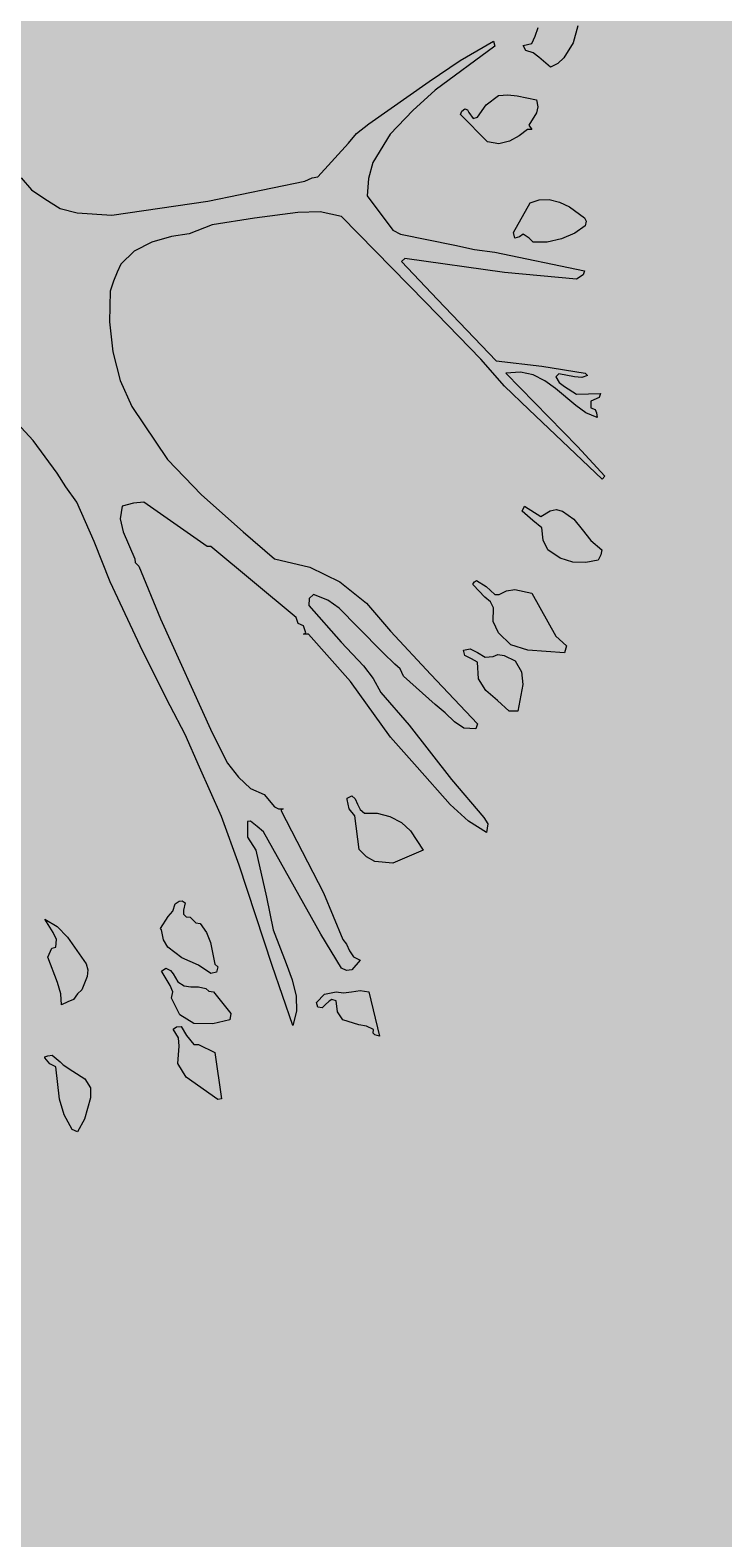
# Model space of a CAD drawing. Units: inches. Extents: x 84 to 1044, y -280 to 906.
# Tile 58 of 105: x 401.24 to 411.62, y 738.5 to 761.07. Entities that reach past the tile are written whole.
import ezdxf

# ---------------------------------------------------------------- set-up
doc = ezdxf.new("R2010")
doc.units = ezdxf.units.IN
doc.layers.add('A-ANNO-DIMS', color=2, linetype='Continuous', lineweight=18)
doc.layers.add('L-PLNT', color=114, linetype='Continuous', lineweight=15)
doc.layers.add('L-PLNT-PATT', color=9, linetype='Continuous', lineweight=9, true_color=0xafd9aa)
doc.styles.get("Standard").update_dxf_attribs({"font": 'arial.ttf'})
doc.dimstyles.get("Standard").update_dxf_attribs({"dimtxt": 0.18, "dimasz": 0.18, "dimexe": 0.18, "dimexo": 0.0625, "dimgap": 0.09, "dimtad": 0, "dimtih": 1, "dimtoh": 1, "dimdec": 4, "dimzin": 0, "dimdsep": 46, "dimtxsty": 'Standard', "dimcen": 0.09, "dimadec": 0, "dimazin": 0, "dimtfac": 1, "dimtdec": 4, "dimtofl": 0, "dimtmove": 0, "dimatfit": 3, "dimfxl": 1, "dimtolj": 1, "dimtzin": 0, "dimarcsym": 0})

# ---------------------------------------------------------------- blocks, each defined once
blk = doc.blocks.new('A$C37E508DF')
for p, q in [((1.3455, 1.0934), (1.3485, 1.102)), ((1.3875, 1.1037), (1.3828, 1.087)), ((1.2713, 1.0694), (1.3044, 1.0887)), ((1.3044, 1.0887), (1.3057, 1.0835)), ((1.3335, 1.0844), (1.3421, 1.0861)), ((1.3421, 1.0861), (1.3455, 1.0934)), ((1.3828, 1.087), (1.3738, 1.072)), ((1.3057, 1.0835), (1.2469, 1.0402)), ((1.3361, 1.0793), (1.3335, 1.0844)), ((1.3434, 1.0771), (1.3361, 1.0793)), ((1.349, 1.0728), (1.3434, 1.0771)), ((1.3605, 1.063), (1.349, 1.0728)), ((1.3738, 1.072), (1.3678, 1.0664)), ((1.2409, 1.0488), (1.2713, 1.0694)), ((1.3678, 1.0664), (1.3605, 1.063)), ((1.1813, 1.0072), (1.2409, 1.0488)), ((1.2469, 1.0402), (1.2246, 1.0201)), ((1.2885, 1.0136), (1.2971, 1.0257)), ((1.2971, 1.0257), (1.3091, 1.0351)), ((1.3091, 1.0351), (1.3185, 1.0355)), ((1.3185, 1.0355), (1.3275, 1.0347)), ((1.3275, 1.0347), (1.3468, 1.0308)), ((1.3468, 1.0308), (1.3481, 1.0239)), ((1.2246, 1.0201), (1.2023, 0.9969)), ((1.2718, 1.0162), (1.2731, 1.0197)), ((1.2984, 0.9892), (1.2718, 1.0162)), ((1.2731, 1.0197), (1.2761, 1.0218)), ((1.2761, 1.0218), (1.2786, 1.0209)), ((1.2786, 1.0209), (1.2799, 1.0184)), ((1.2799, 1.0184), (1.2842, 1.0124)), ((1.2842, 1.0124), (1.2885, 1.0136)), ((1.3468, 1.018), (1.3391, 1.0059)), ((1.3481, 1.0239), (1.3468, 1.018)), ((1.1612, 0.9879), (1.1693, 0.9974)), ((1.1693, 0.9974), (1.1813, 1.0072)), ((1.2023, 0.9969), (1.1852, 0.9691)), ((1.3378, 1.0016), (1.3297, 0.9952)), ((1.3421, 1.0016), (1.3378, 1.0016)), ((1.3391, 1.0059), (1.3421, 1.0016)), ((1.1311, 0.9549), (1.1612, 0.9879)), ((1.3095, 0.9875), (1.2984, 0.9892)), ((1.3202, 0.9901), (1.3095, 0.9875)), ((1.3297, 0.9952), (1.3202, 0.9901)), ((1.1852, 0.9691), (1.1809, 0.9532)), ((0.8383, 0.954), (0.8486, 0.942)), ((1.1183, 0.9506), (1.1256, 0.954)), ((1.1256, 0.954), (1.1311, 0.9549)), ((1.1809, 0.9532), (1.1796, 0.936)), ((0.8486, 0.942), (0.8619, 0.933)), ((1.0227, 0.9309), (1.1183, 0.9506)), ((0.8619, 0.933), (0.8769, 0.9236)), ((0.8769, 0.9236), (0.8936, 0.9193)), ((0.9279, 0.9172), (1.0227, 0.9309)), ((1.1796, 0.936), (1.2049, 0.9022)), ((1.3241, 0.9), (1.3404, 0.9292)), ((1.3404, 0.9292), (1.3494, 0.9322)), ((1.3494, 0.9322), (1.3592, 0.9326)), ((1.3592, 0.9326), (1.3695, 0.93)), ((1.3695, 0.93), (1.3794, 0.9253)), ((1.3794, 0.9253), (1.394, 0.9146)), ((0.8936, 0.9193), (0.9279, 0.9172)), ((1.0269, 0.9077), (1.0042, 0.8987)), ((1.0685, 0.9142), (1.0269, 0.9077)), ((1.1114, 0.9198), (1.0685, 0.9142)), ((1.1333, 0.9202), (1.1114, 0.9198)), ((1.1543, 0.9159), (1.1333, 0.9202)), ((1.2371, 0.8314), (1.1543, 0.9159)), ((1.3948, 0.9065), (1.3846, 0.8992)), ((1.394, 0.9146), (1.3957, 0.9112)), ((1.3957, 0.9112), (1.3948, 0.9065)), ((0.9866, 0.8962), (0.9673, 0.8906)), ((1.0042, 0.8987), (0.9866, 0.8962)), ((1.2049, 0.9022), (1.2126, 0.8983)), ((1.2126, 0.8983), (1.2662, 0.8876)), ((1.3254, 0.8944), (1.3241, 0.9)), ((1.3301, 0.8957), (1.3254, 0.8944)), ((1.3335, 0.8983), (1.3301, 0.8957)), ((1.3395, 0.8944), (1.3335, 0.8983)), ((1.3434, 0.8906), (1.3395, 0.8944)), ((1.3713, 0.8936), (1.3571, 0.8906)), ((1.3846, 0.8992), (1.3713, 0.8936)), ((0.9498, 0.8816), (0.9369, 0.8687)), ((0.9673, 0.8906), (0.9498, 0.8816)), ((1.2662, 0.8876), (1.2855, 0.8833)), ((1.2855, 0.8833), (1.3057, 0.8807)), ((1.3057, 0.8807), (1.394, 0.8623)), ((1.3571, 0.8906), (1.3434, 0.8906)), ((0.9369, 0.8687), (0.933, 0.861)), ((1.2169, 0.8743), (1.2135, 0.8713)), ((1.2135, 0.8713), (1.2491, 0.834)), ((1.3151, 0.8606), (1.2169, 0.8743)), ((1.394, 0.8623), (1.3927, 0.8584)), ((0.9296, 0.852), (0.9262, 0.8421)), ((0.933, 0.861), (0.9296, 0.852)), ((1.3863, 0.8541), (1.3151, 0.8606)), ((1.3927, 0.8584), (1.3863, 0.8541)), ((0.9262, 0.8421), (0.9257, 0.8121)), ((1.2491, 0.834), (1.3069, 0.7735)), ((1.2919, 0.7752), (1.2371, 0.8314)), ((0.9257, 0.8121), (0.9287, 0.7825)), ((0.9287, 0.7825), (0.936, 0.7542)), ((1.3151, 0.7487), (1.2919, 0.7752)), ((1.3069, 0.7735), (1.352, 0.7684)), ((1.3309, 0.7624), (1.3164, 0.7615)), ((1.3164, 0.7615), (1.3871, 0.6891)), ((1.3434, 0.7598), (1.3309, 0.7624)), ((1.355, 0.7538), (1.3434, 0.7598)), ((1.352, 0.7684), (1.3948, 0.7615)), ((1.3687, 0.7607), (1.3657, 0.7577)), ((1.3841, 0.7577), (1.3687, 0.7607)), ((1.397, 0.759), (1.3914, 0.7572)), ((1.3948, 0.7615), (1.397, 0.759)), ((0.936, 0.7542), (0.9476, 0.7285)), ((1.3391, 0.7255), (1.3151, 0.7487)), ((1.3653, 0.7461), (1.355, 0.7538)), ((1.3854, 0.7294), (1.3653, 0.7461)), ((1.3657, 0.7577), (1.3691, 0.7521)), ((1.3691, 0.7521), (1.3743, 0.7482)), ((1.3743, 0.7482), (1.3863, 0.7405)), ((1.3914, 0.7572), (1.3841, 0.7577)), ((0.9476, 0.7285), (0.9828, 0.6762)), ((1.3953, 0.7221), (1.3854, 0.7294)), ((1.3863, 0.7405), (1.4099, 0.7414)), ((1.4086, 0.7375), (1.4004, 0.7337)), ((1.4004, 0.7337), (1.4004, 0.7272)), ((1.4099, 0.7414), (1.4086, 0.7375)), ((1.4116, 0.6569), (1.3391, 0.7255)), ((1.4064, 0.7178), (1.3953, 0.7221)), ((1.4004, 0.7272), (1.4047, 0.7255)), ((1.4047, 0.7255), (1.406, 0.7221)), ((1.406, 0.7221), (1.4064, 0.7178)), ((0.8503, 0.6951), (0.8344, 0.7122)), ((0.8739, 0.6629), (0.8503, 0.6951)), ((1.3871, 0.6891), (1.4141, 0.6599)), ((0.9828, 0.6762), (1.0162, 0.6415)), ((0.8824, 0.6492), (0.8739, 0.6629)), ((1.4141, 0.6599), (1.4116, 0.6569)), ((0.8932, 0.6342), (0.8824, 0.6492)), ((1.0162, 0.6415), (1.0574, 0.605)), ((0.9103, 0.5956), (0.8932, 0.6342)), ((0.9382, 0.6303), (0.936, 0.6179)), ((0.9493, 0.6333), (0.9382, 0.6303)), ((0.9596, 0.6342), (0.9493, 0.6333)), ((1.0218, 0.5904), (0.9596, 0.6342)), ((1.3327, 0.6252), (1.3348, 0.6303)), ((1.343, 0.6162), (1.3327, 0.6252)), ((1.3348, 0.6303), (1.3511, 0.62)), ((1.3511, 0.62), (1.3601, 0.6256)), ((1.3601, 0.6256), (1.3661, 0.6269)), ((1.3661, 0.6269), (1.3725, 0.6252)), ((1.3725, 0.6252), (1.3837, 0.6175)), ((0.936, 0.6179), (0.939, 0.605)), ((1.352, 0.6089), (1.343, 0.6162)), ((1.3837, 0.6175), (1.3918, 0.6072)), ((0.9262, 0.5557), (0.9103, 0.5956)), ((0.939, 0.605), (0.9506, 0.5784)), ((1.0574, 0.605), (1.0883, 0.5784)), ((1.3533, 0.5969), (1.352, 0.6089)), ((1.358, 0.5874), (1.3533, 0.5969)), ((1.3918, 0.6072), (1.4004, 0.5964)), ((1.4004, 0.5964), (1.4111, 0.5874)), ((1.0256, 0.5904), (1.0218, 0.5904)), ((1.1097, 0.5205), (1.0256, 0.5904)), ((1.37, 0.5789), (1.358, 0.5874)), ((1.4103, 0.5823), (1.4077, 0.5771)), ((1.4111, 0.5874), (1.4103, 0.5823)), ((0.9506, 0.5784), (0.951, 0.5746)), ((0.951, 0.5746), (0.9545, 0.5711)), ((0.9545, 0.5711), (0.9759, 0.5193)), ((1.0883, 0.5784), (1.123, 0.5703)), ((1.123, 0.5703), (1.1526, 0.5557)), ((1.3824, 0.575), (1.37, 0.5789)), ((1.3953, 0.5746), (1.3824, 0.575)), ((1.4077, 0.5771), (1.3953, 0.5746)), ((0.9583, 0.4871), (0.9262, 0.5557)), ((1.1526, 0.5557), (1.1792, 0.5347)), ((1.2842, 0.554), (1.2855, 0.5557)), ((1.2842, 0.5527), (1.2842, 0.554)), ((1.2958, 0.5407), (1.2842, 0.5527)), ((1.2855, 0.5557), (1.2876, 0.557)), ((1.2876, 0.557), (1.2971, 0.551)), ((1.2971, 0.551), (1.3057, 0.5433)), ((1.1226, 0.5394), (1.1221, 0.5325)), ((1.1268, 0.5433), (1.1226, 0.5394)), ((1.141, 0.5377), (1.1268, 0.5433)), ((1.1521, 0.5296), (1.141, 0.5377)), ((1.3014, 0.536), (1.2958, 0.5407)), ((1.3044, 0.53), (1.3014, 0.536)), ((1.3057, 0.5433), (1.3099, 0.5433)), ((1.3099, 0.5433), (1.3172, 0.5467)), ((1.3172, 0.5467), (1.3254, 0.548)), ((1.3254, 0.548), (1.3421, 0.5446)), ((1.3421, 0.5446), (1.3657, 0.5021)), ((1.1118, 0.5145), (1.1097, 0.5205)), ((1.1221, 0.5325), (1.1539, 0.4961)), ((1.1706, 0.5111), (1.1521, 0.5296)), ((1.1792, 0.5347), (1.2027, 0.5072)), ((1.3039, 0.5167), (1.3044, 0.53)), ((0.9759, 0.5193), (1.0269, 0.4069)), ((1.117, 0.5124), (1.1118, 0.5145)), ((1.1191, 0.5055), (1.117, 0.5124)), ((1.117, 0.5042), (1.1191, 0.5055)), ((1.1955, 0.4858), (1.1706, 0.5111)), ((1.2027, 0.5072), (1.2426, 0.4644)), ((1.3091, 0.5055), (1.3039, 0.5167)), ((1.3215, 0.4935), (1.3091, 0.5055)), ((1.1217, 0.5042), (1.117, 0.5042)), ((1.1633, 0.4575), (1.1217, 0.5042)), ((1.1539, 0.4961), (1.1762, 0.4729)), ((1.3382, 0.4884), (1.3215, 0.4935)), ((1.3657, 0.5021), (1.3764, 0.4927)), ((1.3764, 0.4927), (1.3743, 0.4858)), ((0.9853, 0.4335), (0.9583, 0.4871)), ((1.207, 0.4747), (1.1955, 0.4858)), ((1.2748, 0.4884), (1.2812, 0.4897)), ((1.2761, 0.4832), (1.2748, 0.4884)), ((1.2825, 0.4798), (1.2761, 0.4832)), ((1.2812, 0.4897), (1.2885, 0.4862)), ((1.2885, 0.4764), (1.2825, 0.4798)), ((1.2885, 0.4862), (1.2962, 0.4815)), ((1.2894, 0.4601), (1.2885, 0.4764)), ((1.2962, 0.4815), (1.3039, 0.482)), ((1.3039, 0.482), (1.3087, 0.4841)), ((1.3087, 0.4841), (1.3147, 0.4832)), ((1.3147, 0.4832), (1.3258, 0.4777)), ((1.3258, 0.4777), (1.3318, 0.4669)), ((1.3743, 0.4858), (1.3382, 0.4884)), ((1.1762, 0.4729), (1.1856, 0.4605)), ((1.2122, 0.47), (1.207, 0.4747)), ((1.2156, 0.4627), (1.2122, 0.47)), ((1.2469, 0.4348), (1.2156, 0.4627)), ((1.2426, 0.4644), (1.2885, 0.4159)), ((1.3318, 0.4669), (1.3331, 0.4545)), ((1.2027, 0.4026), (1.1633, 0.4575)), ((1.1856, 0.4605), (1.1933, 0.4468)), ((1.1933, 0.4468), (1.2212, 0.4146)), ((1.2967, 0.4485), (1.2894, 0.4601)), ((1.3082, 0.4386), (1.2967, 0.4485)), ((1.3331, 0.4545), (1.3284, 0.4284)), ((1.0003, 0.4052), (0.9853, 0.4335)), ((1.2568, 0.4266), (1.2469, 0.4348)), ((1.3198, 0.4284), (1.3082, 0.4386)), ((1.2658, 0.4176), (1.2568, 0.4266)), ((1.2752, 0.4116), (1.2658, 0.4176)), ((1.3284, 0.4284), (1.3198, 0.4284)), ((1.0145, 0.373), (1.0003, 0.4052)), ((1.0269, 0.4069), (1.0419, 0.3769)), ((1.2289, 0.373), (1.2027, 0.4026)), ((1.2212, 0.4146), (1.2628, 0.361)), ((1.2868, 0.4108), (1.2752, 0.4116)), ((1.2885, 0.4159), (1.2868, 0.4108)), ((1.0359, 0.3246), (1.0145, 0.373)), ((1.0419, 0.3769), (1.0527, 0.3632)), ((1.2615, 0.3362), (1.2289, 0.373)), ((1.0527, 0.3632), (1.0647, 0.352)), ((1.2628, 0.361), (1.2949, 0.3233)), ((1.0647, 0.352), (1.078, 0.346)), ((1.078, 0.346), (1.0883, 0.334)), ((1.1599, 0.3426), (1.1646, 0.3447)), ((1.1599, 0.3413), (1.1599, 0.3426)), ((1.1646, 0.3447), (1.168, 0.3417)), ((1.0883, 0.334), (1.0921, 0.3319)), ((1.0921, 0.3319), (1.0968, 0.3319)), ((1.0968, 0.3319), (1.0947, 0.3306)), ((1.0947, 0.3306), (1.1367, 0.2491)), ((1.162, 0.3319), (1.1599, 0.3413)), ((1.1676, 0.325), (1.162, 0.3319)), ((1.168, 0.3417), (1.1702, 0.3366)), ((1.1702, 0.3366), (1.1727, 0.3314)), ((1.1727, 0.3314), (1.177, 0.3276)), ((1.177, 0.3276), (1.1895, 0.3276)), ((1.1895, 0.3276), (1.2019, 0.3246)), ((1.2795, 0.3199), (1.2615, 0.3362)), ((1.0535, 0.2766), (1.0359, 0.3246)), ((1.0647, 0.3199), (1.0617, 0.3194)), ((1.0617, 0.3194), (1.0617, 0.304)), ((1.0711, 0.3147), (1.0647, 0.3199)), ((1.0775, 0.3092), (1.0711, 0.3147)), ((1.1719, 0.292), (1.1676, 0.325)), ((1.2019, 0.3246), (1.2135, 0.3186)), ((1.2135, 0.3186), (1.2225, 0.3104)), ((1.2975, 0.3087), (1.2795, 0.3199)), ((1.2949, 0.3233), (1.2988, 0.3173)), ((1.2988, 0.3173), (1.2975, 0.3087)), ((1.0617, 0.304), (1.0698, 0.2911)), ((1.1341, 0.2084), (1.0775, 0.3092)), ((1.2225, 0.3104), (1.2349, 0.2911)), ((1.0698, 0.2911), (1.0805, 0.2448)), ((1.1792, 0.2847), (1.1719, 0.292)), ((1.1873, 0.28), (1.1792, 0.2847)), ((1.2349, 0.2911), (1.2049, 0.2783)), ((1.0861, 0.1775), (1.0535, 0.2766)), ((1.2049, 0.2783), (1.1873, 0.28)), ((0.9879, 0.2311), (0.9905, 0.2384)), ((0.9905, 0.2384), (0.9943, 0.241)), ((0.9943, 0.241), (0.9973, 0.2414)), ((0.9973, 0.2414), (1.0003, 0.2393)), ((1.0003, 0.2393), (0.9986, 0.232)), ((1.0805, 0.2448), (1.087, 0.2127)), ((1.1367, 0.2491), (1.1556, 0.2032)), ((0.8619, 0.2234), (0.8739, 0.2161)), ((0.87, 0.2101), (0.8619, 0.2234)), ((0.9759, 0.214), (0.9836, 0.226)), ((0.9836, 0.226), (0.9879, 0.2311)), ((0.9986, 0.232), (0.9986, 0.2281)), ((0.9986, 0.2281), (1.0012, 0.2255)), ((1.0012, 0.2255), (1.0051, 0.2251)), ((1.0051, 0.2251), (1.0076, 0.2225)), ((0.8734, 0.2032), (0.87, 0.2101)), ((0.8739, 0.2161), (0.8841, 0.2054)), ((0.9768, 0.2127), (0.9759, 0.214)), ((0.9789, 0.2028), (0.9768, 0.2127)), ((1.0076, 0.2225), (1.0106, 0.2195)), ((1.0106, 0.2195), (1.0149, 0.2191)), ((1.0149, 0.2191), (1.0214, 0.2101)), ((1.0214, 0.2101), (1.0252, 0.2002)), ((1.087, 0.2127), (1.0998, 0.1797)), ((1.1543, 0.1749), (1.1341, 0.2084)), ((0.8649, 0.1857), (0.8687, 0.1947)), ((0.8687, 0.1947), (0.8726, 0.1955)), ((0.8726, 0.1955), (0.8734, 0.2032)), ((0.8841, 0.2054), (0.9026, 0.1792)), ((0.9832, 0.1955), (0.9789, 0.2028)), ((0.9969, 0.1852), (0.9832, 0.1955)), ((1.0252, 0.2002), (1.0295, 0.1788)), ((1.1556, 0.2032), (1.1594, 0.1985)), ((1.1594, 0.1985), (1.1624, 0.1921)), ((0.8743, 0.1608), (0.8649, 0.1857)), ((0.9026, 0.1792), (0.9043, 0.1732)), ((1.0132, 0.1779), (0.9969, 0.1852)), ((1.0295, 0.1788), (1.0325, 0.1762)), ((1.0998, 0.1797), (1.1058, 0.1634)), ((1.1624, 0.1921), (1.1663, 0.1861)), ((1.1727, 0.1827), (1.1646, 0.1732)), ((1.1663, 0.1861), (1.1727, 0.1827)), ((0.9035, 0.1668), (0.8983, 0.1535)), ((0.9043, 0.1732), (0.9035, 0.1668)), ((0.9768, 0.1719), (0.9811, 0.1749)), ((0.9776, 0.1711), (0.9768, 0.1719)), ((0.9853, 0.1578), (0.9776, 0.1711)), ((0.9811, 0.1749), (0.9858, 0.1728)), ((0.9858, 0.1728), (0.9884, 0.1694)), ((0.9884, 0.1694), (0.9931, 0.1616)), ((1.0256, 0.1698), (1.0132, 0.1779)), ((1.0312, 0.1711), (1.0256, 0.1698)), ((1.0325, 0.1762), (1.0312, 0.1711)), ((1.1063, 0.1183), (1.0861, 0.1775)), ((1.1594, 0.1728), (1.1543, 0.1749)), ((1.1646, 0.1732), (1.1594, 0.1728)), ((0.8777, 0.1496), (0.8743, 0.1608)), ((0.8781, 0.1389), (0.8777, 0.1496)), ((0.894, 0.1496), (0.8902, 0.1441)), ((0.8983, 0.1535), (0.894, 0.1496)), ((0.9879, 0.1518), (0.9853, 0.1578)), ((0.9866, 0.1453), (0.9879, 0.1518)), ((0.9931, 0.1616), (0.9991, 0.1574)), ((0.9991, 0.1574), (1.0059, 0.1565)), ((1.0059, 0.1565), (1.0132, 0.1565)), ((1.0132, 0.1565), (1.0205, 0.1548)), ((1.0205, 0.1548), (1.0235, 0.1522)), ((1.0235, 0.1522), (1.0282, 0.1518)), ((1.0282, 0.1518), (1.0454, 0.1303)), ((1.1058, 0.1634), (1.1097, 0.1475)), ((1.1298, 0.1411), (1.1376, 0.1492)), ((1.1376, 0.1492), (1.1491, 0.1518)), ((1.1491, 0.1518), (1.1564, 0.1505)), ((1.1564, 0.1505), (1.1642, 0.1518)), ((1.1642, 0.1518), (1.1727, 0.1531)), ((1.1727, 0.1531), (1.1813, 0.1518)), ((1.1813, 0.1518), (1.192, 0.108)), ((0.8846, 0.1419), (0.8781, 0.1389)), ((0.8902, 0.1441), (0.8846, 0.1419)), ((0.9948, 0.1291), (0.9866, 0.1453)), ((1.1097, 0.1475), (1.1101, 0.1325)), ((1.1311, 0.1364), (1.1298, 0.1411)), ((1.1354, 0.1359), (1.1311, 0.1364)), ((1.1384, 0.1389), (1.1354, 0.1359)), ((1.1423, 0.1423), (1.1384, 0.1389)), ((1.1449, 0.1441), (1.1423, 0.1423)), ((1.1491, 0.1428), (1.1449, 0.1441)), ((1.1504, 0.132), (1.1491, 0.1428)), ((1.0089, 0.1205), (0.9948, 0.1291)), ((1.0274, 0.12), (1.0089, 0.1205)), ((1.0441, 0.1239), (1.0274, 0.12)), ((1.0454, 0.1303), (1.0441, 0.1239)), ((1.1101, 0.1325), (1.1063, 0.1183)), ((1.1556, 0.1239), (1.1504, 0.132)), ((1.1714, 0.1192), (1.1556, 0.1239)), ((1.1792, 0.1179), (1.1714, 0.1192)), ((0.9884, 0.1149), (0.9918, 0.117)), ((0.9935, 0.1063), (0.9884, 0.1149)), ((0.9918, 0.117), (0.9961, 0.1175)), ((0.9943, 0.0982), (0.9935, 0.1063)), ((0.9961, 0.1175), (1.0016, 0.1085)), ((1.0016, 0.1085), (1.0089, 0.0999)), ((1.186, 0.1145), (1.1792, 0.1179)), ((1.1856, 0.111), (1.186, 0.1145)), ((1.1873, 0.1093), (1.1856, 0.111)), ((1.192, 0.108), (1.1873, 0.1093)), ((0.8649, 0.0887), (0.8691, 0.0892)), ((0.8691, 0.0892), (0.8769, 0.0827)), ((0.9931, 0.081), (0.9943, 0.0982)), ((1.0089, 0.0999), (1.0132, 0.0999)), ((1.0132, 0.0999), (1.0295, 0.0917)), ((1.0295, 0.0917), (1.0359, 0.0463)), ((0.8619, 0.0875), (0.8649, 0.0887)), ((0.8619, 0.0866), (0.8619, 0.0875)), ((0.8666, 0.0806), (0.8619, 0.0866)), ((0.8726, 0.0776), (0.8666, 0.0806)), ((0.8764, 0.0459), (0.8726, 0.0776)), ((0.8769, 0.0827), (0.8799, 0.0797)), ((0.8799, 0.0797), (0.8893, 0.0733)), ((1.0012, 0.0677), (0.9931, 0.081)), ((0.8893, 0.0733), (0.9013, 0.066)), ((0.9013, 0.066), (0.9069, 0.057)), ((1.0325, 0.0454), (1.0012, 0.0677)), ((0.8807, 0.0304), (0.8764, 0.0459)), ((0.9069, 0.0471), (0.9009, 0.0261)), ((0.9069, 0.057), (0.9069, 0.0471)), ((1.0359, 0.0463), (1.0325, 0.0454)), ((0.8889, 0.0159), (0.8807, 0.0304)), ((0.894, 0.0137), (0.8889, 0.0159)), ((0.9009, 0.0261), (0.894, 0.0137))]:
    blk.add_line(p, q)
blk = doc.blocks.new('*D62')
at = {"layer": 'A-ANNO-DIMS', "color": 0, "lineweight": -2, "transparency": 16777216}
for p, q in [((203.179, 709.183), (203.179, 905.9)), ((896.074, 400.183), (896.074, 905.9)), ((203.359, 905.72), (549.232, 905.72)), ((895.894, 905.72), (550.021, 905.72))]:
    blk.add_line(p, q, dxfattribs=at)
at = {"layer": 'A-ANNO-DIMS', "color": 0, "transparency": 16777216}
for points in [[(203.359, 905.75), (203.359, 905.69), (203.179, 905.72)], [(895.894, 905.75), (895.894, 905.69), (896.074, 905.72)]]:
    blk.add_solid(points, dxfattribs=at)
at = {"layer": 'Defpoints', "color": 0, "transparency": 16777216}
for p in [(896.074, 905.72), (203.179, 709.12), (896.074, 400.12)]:
    blk.add_point(p, dxfattribs=at)
at = {"layer": 'A-ANNO-DIMS', "color": 0, "transparency": 16777216, "insert": (549.627, 905.72), "char_height": 0.18, "attachment_point": 5}
blk.add_mtext('\\A1;692.9', dxfattribs=at)

msp = doc.modelspace()

# ---------------------------------------------------------------- hatches: boundary and pattern name
at = {"layer": 'L-PLNT-PATT', "transparency": 33554597}
h = msp.add_hatch(color=256, dxfattribs=at)
h.dxf.hatch_style = 1
h.paths.add_polyline_path([(434.074, 769.12), (386.074, 769.12), (386.074, 709.12), (434.074, 709.12)])
h.paths.add_polyline_path([(896.074, 847.12), (434.074, 847.12), (434.074, 769.12), (434.074, 709.12), (470.074, 709.12), (506.074, 709.12), (572.074, 709.12), (608.074, 709.12), (698.074, 709.12), (770.074, 709.12), (833.074, 709.12), (896.074, 709.12)])
h.paths.add_polyline_path([(983.074, 847.12), (896.074, 847.12), (896.074, 709.12), (896.074, 547.12), (932.074, 547.12), (983.074, 547.12)])
h.paths.add_polyline_path([(983.074, 547.12), (932.074, 547.12), (932.074, 265.12), (983.074, 265.12)])
h.paths.add_polyline_path([(203.179, 646.12), (203.179, 709.12), (203.179, 745.12), (143.179, 745.12), (143.179, 271.12), (203.179, 271.12), (203.179, 274.12), (203.179, 310.12), (203.179, 574.12)])

# ---------------------------------------------------------------- block references
at = {"layer": 'L-PLNT', "xscale": 15.19586232982809, "yscale": 15.19586232982809, "zscale": 15.19586232982809}
msp.add_blockref('A$C37E508DF', (388.36, 744.368), dxfattribs=at)

# ---------------------------------------------------------------- dimensions: what is measured, and where the dimension line sits
at = {"layer": 'A-ANNO-DIMS'}
dim = msp.add_linear_dim(base=(896.074, 905.72), p1=(203.179, 709.12), p2=(896.074, 400.12), dimstyle='Standard', override={"dimdec": 1, "dimlfac": 1, "dimrnd": 0, "dimzin": 0, "dimdsep": 46, "dimlunit": 2}, dxfattribs=at)
dim.commit()
dim.dimension.update_dxf_attribs({"geometry": '*D62', "text_midpoint": (549.627, 905.72)})

doc.saveas('drawing.dxf')
